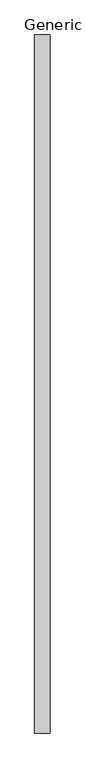
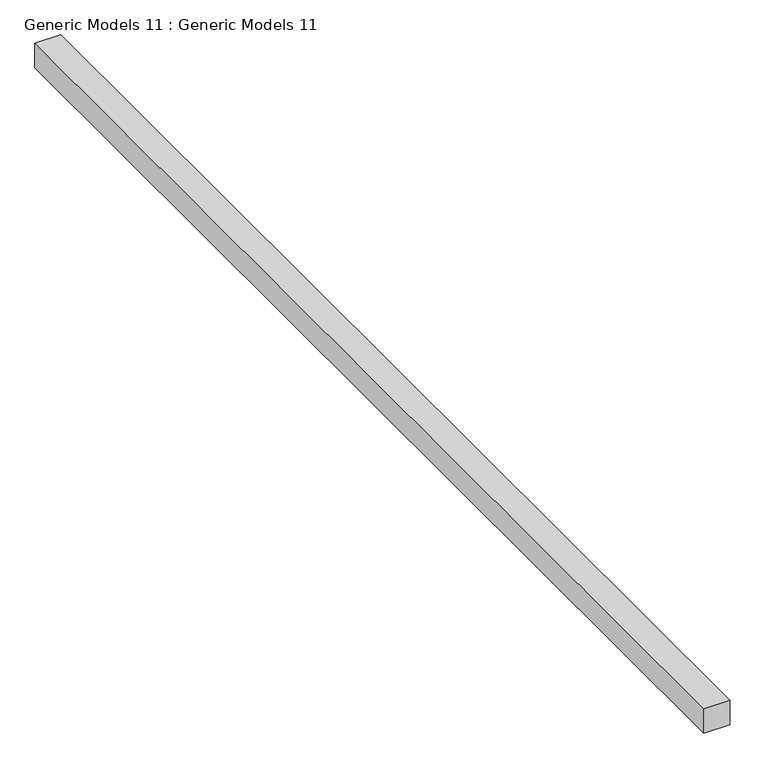
"""IFC4 building model written with IfcOpenShell, lengths in millimetres: proxy geometry, Generic Models 11 : Generic Models 11."""

from ifc_helpers import new_model, si_unit, frame, origin, place, context, project, spatial, polyline, outline, extrude, source, transform, mapped, element, save


def generic_models_11_generic_models_11_f4245121(model_context):
    return source(origin(), model_context, "Body", "SweptSolid", [
        extrude(outline(polyline([(-14138.2638778, 3755.9646462), (-14138.2638778, 17410.2237525), (-13833.4638778, 17410.2237525), (-13833.4638778, 3755.9646462), (-14138.2638778, 3755.9646462)])), frame((0.0, 0.0, 9144.0), z_axis=(0.0, 0.0, 1.0), x_axis=(1.0, 0.0, 0.0)), (0.0, 0.0, 1.0), 304.8),
    ])


if __name__ == "__main__":
    model = new_model("IFC4")
    model_context = context("Model", 3, world=origin())
    ifc_project = project(units=[si_unit("LENGTHUNIT", "METRE", prefix="MILLI")], contexts=[model_context])
    site = spatial("IfcSite", under=ifc_project)
    building = spatial("IfcBuilding", under=site)
    placement = place(None, origin())
    generic_models_11_generic_models_11_shape = generic_models_11_generic_models_11_f4245121(model_context)
    element("IfcBuildingElementProxy", 1, Name="Generic Models 11 : Generic Models 11", ObjectType="Generic Models 11 : Generic Models 11", at=placement, inside=building, context=model_context, shape_type="MappedRepresentation", body=[
        mapped(generic_models_11_generic_models_11_shape, transform((0.0, 0.0, 0.0), x_axis=(1.0, 0.0, 0.0), y_axis=(0.0, 1.0, 0.0), z_axis=(0.0, 0.0, 1.0))),
    ])
    save(model, "model.ifc")
